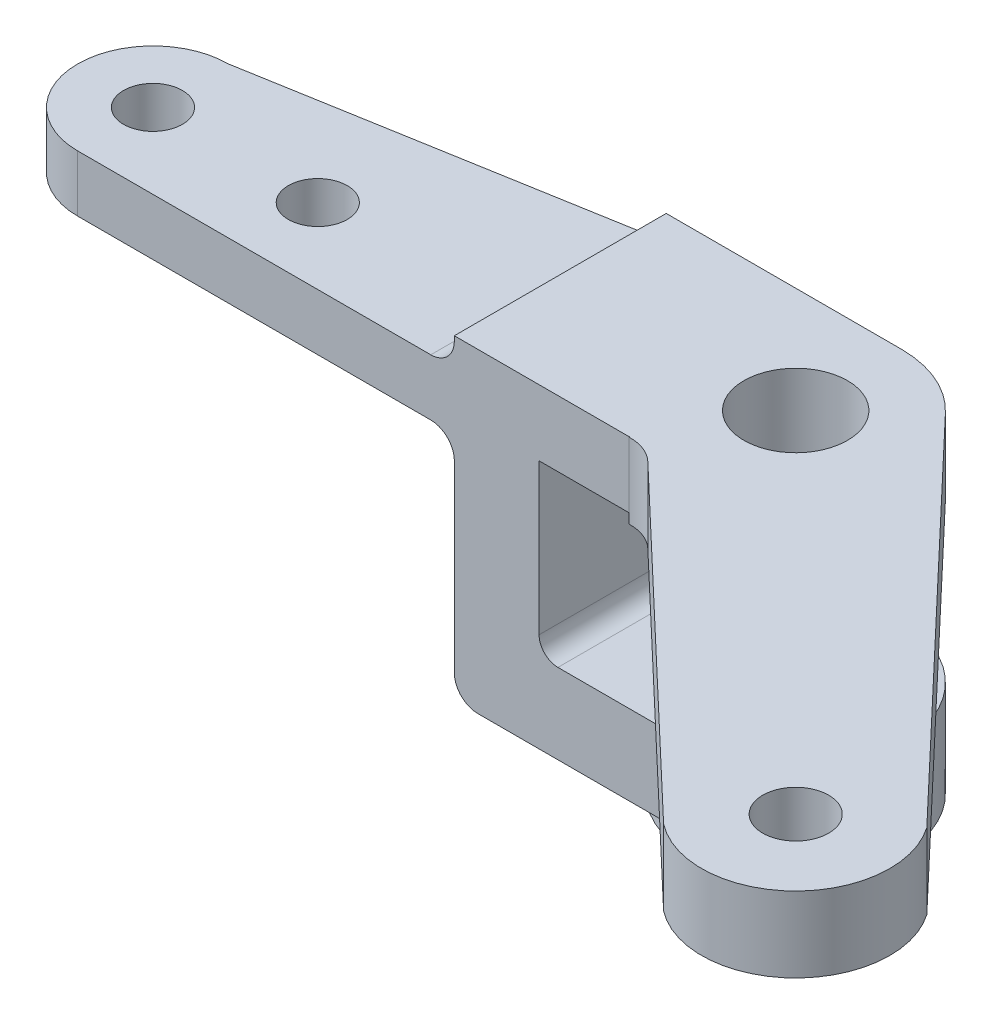
ISO-10303-21;
HEADER;
FILE_DESCRIPTION(('STEP AP214'),'2;1');
FILE_NAME('part.step','',(''),(''),'','','');
FILE_SCHEMA(('AUTOMOTIVE_DESIGN { 1 0 10303 214 1 1 1 1 }'));
ENDSEC;
DATA;
#1=APPLICATION_CONTEXT('core data for automotive mechanical design processes');
#2=APPLICATION_PROTOCOL_DEFINITION('international standard','automotive_design',2000,#1);
#3=PRODUCT_CONTEXT('',#1,'mechanical');
#4=PRODUCT('Part','Part','',(#3));
#5=PRODUCT_RELATED_PRODUCT_CATEGORY('part','',(#4));
#6=PRODUCT_DEFINITION_FORMATION('','',#4);
#7=PRODUCT_DEFINITION_CONTEXT('part definition',#1,'design');
#8=PRODUCT_DEFINITION('design','',#6,#7);
#9=PRODUCT_DEFINITION_SHAPE('','',#8);
#10=(LENGTH_UNIT() NAMED_UNIT(*) SI_UNIT(.MILLI.,.METRE.));
#11=(NAMED_UNIT(*) PLANE_ANGLE_UNIT() SI_UNIT($,.RADIAN.));
#12=(NAMED_UNIT(*) SI_UNIT($,.STERADIAN.) SOLID_ANGLE_UNIT());
#13=UNCERTAINTY_MEASURE_WITH_UNIT(LENGTH_MEASURE(1.E-05),#10,'distance_accuracy_value','');
#14=(GEOMETRIC_REPRESENTATION_CONTEXT(3) GLOBAL_UNCERTAINTY_ASSIGNED_CONTEXT((#13)) GLOBAL_UNIT_ASSIGNED_CONTEXT((#10,
#11,#12)) REPRESENTATION_CONTEXT('',''));
#15=CARTESIAN_POINT('',(0.,0.,0.));
#16=DIRECTION('',(0.,0.,1.));
#17=DIRECTION('',(1.,0.,0.));
#18=AXIS2_PLACEMENT_3D('',#15,#16,#17);
#19=CARTESIAN_POINT('',(130.,-16.,22.5));
#20=DIRECTION('',(0.,1.,0.));
#21=DIRECTION('',(0.,0.,1.));
#22=AXIS2_PLACEMENT_3D('',#19,#20,#21);
#23=PLANE('',#22);
#24=CARTESIAN_POINT('',(204.246212024587,-16.,96.7462120245875));
#25=DIRECTION('',(0.,-1.,0.));
#26=DIRECTION('',(0.,0.,-1.));
#27=AXIS2_PLACEMENT_3D('',#24,#25,#26);
#28=CIRCLE('',#27,6.99999999999999);
#29=CARTESIAN_POINT('',(204.246212024587,-16.,89.7462120245875));
#30=VERTEX_POINT('',#29);
#31=EDGE_CURVE('E445',#30,#30,#28,.T.);
#32=ORIENTED_EDGE('',*,*,#31,.F.);
#33=EDGE_LOOP('',(#32));
#34=FACE_BOUND('',#33,.T.);
#35=CARTESIAN_POINT('',(130.,-16.,22.5));
#36=DIRECTION('',(0.,-1.,0.));
#37=DIRECTION('',(0.,0.,-1.));
#38=AXIS2_PLACEMENT_3D('',#35,#36,#37);
#39=CIRCLE('',#38,22.5);
#40=CARTESIAN_POINT('',(146.71198303914,-16.,7.43482084741492));
#41=VERTEX_POINT('',#40);
#42=CARTESIAN_POINT('',(119.312759657145,-16.,42.2998205510569));
#43=VERTEX_POINT('',#42);
#44=EDGE_CURVE('E200',#41,#43,#39,.T.);
#45=ORIENTED_EDGE('',*,*,#44,.F.);
#46=DIRECTION('',(0.68856588169474,0.,0.725173790595017));
#47=VECTOR('',#46,1.);
#48=CARTESIAN_POINT('',(145.909902576698,-16.,6.5900974233029));
#49=LINE('',#48,#47);
#50=CARTESIAN_POINT('',(220.648460974255,-16.,85.3021642532294));
#51=VERTEX_POINT('',#50);
#52=EDGE_CURVE('E202',#41,#51,#49,.T.);
#53=ORIENTED_EDGE('',*,*,#52,.T.);
#54=CARTESIAN_POINT('',(204.246212024587,-16.,96.746212024588));
#55=DIRECTION('',(0.,-1.,0.));
#56=DIRECTION('',(0.,0.,-1.));
#57=AXIS2_PLACEMENT_3D('',#54,#55,#56);
#58=CIRCLE('',#57,20.);
#59=CARTESIAN_POINT('',(192.010008711411,-16.,112.566304580531));
#60=VERTEX_POINT('',#59);
#61=EDGE_CURVE('E228',#51,#60,#58,.T.);
#62=ORIENTED_EDGE('',*,*,#61,.T.);
#63=DIRECTION('',(-0.724655837018528,0.,-0.689110961946606));
#64=VECTOR('',#63,1.);
#65=CARTESIAN_POINT('',(192.010008711411,-16.,112.566304580531));
#66=LINE('',#65,#64);
#67=CARTESIAN_POINT('',(123.660042494375,-16.,47.5689519577642));
#68=VERTEX_POINT('',#67);
#69=EDGE_CURVE('E226',#60,#68,#66,.T.);
#70=ORIENTED_EDGE('',*,*,#69,.T.);
#71=CARTESIAN_POINT('',(117.458043836856,-16.,54.0908544909309));
#72=DIRECTION('',(0.,1.,0.));
#73=DIRECTION('',(0.,0.,1.));
#74=AXIS2_PLACEMENT_3D('',#71,#72,#73);
#75=CIRCLE('',#74,9.);
#76=CARTESIAN_POINT('',(117.231837637058,-16.,45.0936976758491));
#77=VERTEX_POINT('',#76);
#78=EDGE_CURVE('E229',#68,#77,#75,.T.);
#79=ORIENTED_EDGE('',*,*,#78,.T.);
#80=DIRECTION('',(0.597335430440409,0.,-0.80199151089059));
#81=VECTOR('',#80,1.);
#82=CARTESIAN_POINT('',(117.231837637058,-16.,45.0936976758491));
#83=LINE('',#82,#81);
#84=EDGE_CURVE('E207',#77,#43,#83,.T.);
#85=ORIENTED_EDGE('',*,*,#84,.T.);
#86=EDGE_LOOP('',(#45,#53,#62,#70,#79,#85));
#87=FACE_BOUND('',#86,.T.);
#88=ADVANCED_FACE('F50',(#34,#87),#23,.F.);
#89=CARTESIAN_POINT('',(80.,-50.,45.));
#90=DIRECTION('',(1.,0.,0.));
#91=DIRECTION('',(0.,0.,-1.));
#92=AXIS2_PLACEMENT_3D('',#89,#90,#91);
#93=PLANE('',#92);
#94=DIRECTION('',(0.,-1.,0.));
#95=VECTOR('',#94,1.);
#96=CARTESIAN_POINT('',(80.,-50.,0.));
#97=LINE('',#96,#95);
#98=CARTESIAN_POINT('',(80.,0.,0.));
#99=VERTEX_POINT('',#98);
#100=CARTESIAN_POINT('',(80.,-0.999999999999966,0.));
#101=VERTEX_POINT('',#100);
#102=EDGE_CURVE('E344',#99,#101,#97,.T.);
#103=ORIENTED_EDGE('',*,*,#102,.T.);
#104=DIRECTION('',(0.,0.,1.));
#105=VECTOR('',#104,1.);
#106=CARTESIAN_POINT('',(80.,-0.999999999999964,0.));
#107=LINE('',#106,#105);
#108=CARTESIAN_POINT('',(80.,-0.999999999999966,45.));
#109=VERTEX_POINT('',#108);
#110=EDGE_CURVE('E296',#101,#109,#107,.T.);
#111=ORIENTED_EDGE('',*,*,#110,.T.);
#112=DIRECTION('',(0.,-1.,0.));
#113=VECTOR('',#112,1.);
#114=CARTESIAN_POINT('',(80.,0.,45.));
#115=LINE('',#114,#113);
#116=CARTESIAN_POINT('',(80.,0.,45.));
#117=VERTEX_POINT('',#116);
#118=EDGE_CURVE('E321',#117,#109,#115,.T.);
#119=ORIENTED_EDGE('',*,*,#118,.F.);
#120=DIRECTION('',(0.,0.,-1.));
#121=VECTOR('',#120,1.);
#122=CARTESIAN_POINT('',(80.,0.,45.));
#123=LINE('',#122,#121);
#124=EDGE_CURVE('E11',#117,#99,#123,.T.);
#125=ORIENTED_EDGE('',*,*,#124,.T.);
#126=EDGE_LOOP('',(#103,#111,#119,#125));
#127=FACE_BOUND('',#126,.T.);
#128=ADVANCED_FACE('F414',(#127),#93,.F.);
#129=CARTESIAN_POINT('',(85.,-67.,45.));
#130=DIRECTION('',(0.,1.,0.));
#131=DIRECTION('',(0.,0.,1.));
#132=AXIS2_PLACEMENT_3D('',#129,#130,#131);
#133=PLANE('',#132);
#134=CARTESIAN_POINT('',(130.,-67.,22.5));
#135=DIRECTION('',(0.,-1.,0.));
#136=DIRECTION('',(0.,0.,-1.));
#137=AXIS2_PLACEMENT_3D('',#134,#135,#136);
#138=CIRCLE('',#137,22.5);
#139=CARTESIAN_POINT('',(130.,-67.,45.));
#140=VERTEX_POINT('',#139);
#141=CARTESIAN_POINT('',(130.,-67.,0.));
#142=VERTEX_POINT('',#141);
#143=EDGE_CURVE('E310',#140,#142,#138,.T.);
#144=ORIENTED_EDGE('',*,*,#143,.F.);
#145=DIRECTION('',(1.,0.,0.));
#146=VECTOR('',#145,1.);
#147=CARTESIAN_POINT('',(85.,-67.,45.));
#148=LINE('',#147,#146);
#149=CARTESIAN_POINT('',(85.,-67.,45.));
#150=VERTEX_POINT('',#149);
#151=EDGE_CURVE('E327',#150,#140,#148,.T.);
#152=ORIENTED_EDGE('',*,*,#151,.F.);
#153=DIRECTION('',(0.,0.,-1.));
#154=VECTOR('',#153,1.);
#155=CARTESIAN_POINT('',(85.,-67.,45.));
#156=LINE('',#155,#154);
#157=CARTESIAN_POINT('',(85.,-67.,0.));
#158=VERTEX_POINT('',#157);
#159=EDGE_CURVE('E367',#150,#158,#156,.T.);
#160=ORIENTED_EDGE('',*,*,#159,.T.);
#161=DIRECTION('',(1.,0.,0.));
#162=VECTOR('',#161,1.);
#163=CARTESIAN_POINT('',(85.,-67.,0.));
#164=LINE('',#163,#162);
#165=EDGE_CURVE('E346',#158,#142,#164,.T.);
#166=ORIENTED_EDGE('',*,*,#165,.T.);
#167=EDGE_LOOP('',(#144,#152,#160,#166));
#168=FACE_BOUND('',#167,.T.);
#169=ADVANCED_FACE('F388',(#168),#133,.F.);
#170=CARTESIAN_POINT('',(80.,0.,45.));
#171=DIRECTION('',(0.,-1.,0.));
#172=DIRECTION('',(0.,0.,-1.));
#173=AXIS2_PLACEMENT_3D('',#170,#171,#172);
#174=PLANE('',#173);
#175=CARTESIAN_POINT('',(130.,0.,22.5));
#176=DIRECTION('',(0.,-1.,0.));
#177=DIRECTION('',(0.,0.,-1.));
#178=AXIS2_PLACEMENT_3D('',#175,#176,#177);
#179=CIRCLE('',#178,11.);
#180=CARTESIAN_POINT('',(130.,0.,11.5));
#181=VERTEX_POINT('',#180);
#182=EDGE_CURVE('E444',#181,#181,#179,.T.);
#183=ORIENTED_EDGE('',*,*,#182,.T.);
#184=EDGE_LOOP('',(#183));
#185=FACE_BOUND('',#184,.T.);
#186=CARTESIAN_POINT('',(204.246212024587,0.,96.7462120245875));
#187=DIRECTION('',(0.,-1.,0.));
#188=DIRECTION('',(0.,0.,-1.));
#189=AXIS2_PLACEMENT_3D('',#186,#187,#188);
#190=CIRCLE('',#189,6.99999999999999);
#191=CARTESIAN_POINT('',(204.246212024587,0.,89.7462120245875));
#192=VERTEX_POINT('',#191);
#193=EDGE_CURVE('E208',#192,#192,#190,.T.);
#194=ORIENTED_EDGE('',*,*,#193,.T.);
#195=EDGE_LOOP('',(#194));
#196=FACE_BOUND('',#195,.T.);
#197=DIRECTION('',(-1.,0.,0.));
#198=VECTOR('',#197,1.);
#199=CARTESIAN_POINT('',(80.,0.,45.));
#200=LINE('',#199,#198);
#201=CARTESIAN_POINT('',(117.301625085896,0.,45.));
#202=VERTEX_POINT('',#201);
#203=EDGE_CURVE('E320',#202,#117,#200,.T.);
#204=ORIENTED_EDGE('',*,*,#203,.F.);
#205=DIRECTION('',(0.597335430440409,0.,-0.80199151089059));
#206=VECTOR('',#205,1.);
#207=CARTESIAN_POINT('',(117.231837637058,0.,45.0936976758491));
#208=LINE('',#207,#206);
#209=CARTESIAN_POINT('',(117.231837637058,0.,45.0936976758491));
#210=VERTEX_POINT('',#209);
#211=EDGE_CURVE('E425',#210,#202,#208,.T.);
#212=ORIENTED_EDGE('',*,*,#211,.F.);
#213=CARTESIAN_POINT('',(117.458043836856,0.,54.0908544909309));
#214=DIRECTION('',(0.,1.,0.));
#215=DIRECTION('',(0.,0.,1.));
#216=AXIS2_PLACEMENT_3D('',#213,#214,#215);
#217=CIRCLE('',#216,9.);
#218=CARTESIAN_POINT('',(123.660042494375,0.,47.5689519577642));
#219=VERTEX_POINT('',#218);
#220=EDGE_CURVE('E236',#219,#210,#217,.T.);
#221=ORIENTED_EDGE('',*,*,#220,.F.);
#222=DIRECTION('',(-0.724655837018528,0.,-0.689110961946606));
#223=VECTOR('',#222,1.);
#224=CARTESIAN_POINT('',(192.010008711411,0.,112.566304580531));
#225=LINE('',#224,#223);
#226=CARTESIAN_POINT('',(192.010008711411,0.,112.566304580531));
#227=VERTEX_POINT('',#226);
#228=EDGE_CURVE('E244',#227,#219,#225,.T.);
#229=ORIENTED_EDGE('',*,*,#228,.F.);
#230=CARTESIAN_POINT('',(204.246212024587,0.,96.746212024588));
#231=DIRECTION('',(0.,-1.,0.));
#232=DIRECTION('',(0.,0.,-1.));
#233=AXIS2_PLACEMENT_3D('',#230,#231,#232);
#234=CIRCLE('',#233,20.);
#235=CARTESIAN_POINT('',(220.648460974255,0.,85.3021642532294));
#236=VERTEX_POINT('',#235);
#237=EDGE_CURVE('E429',#236,#227,#234,.T.);
#238=ORIENTED_EDGE('',*,*,#237,.F.);
#239=DIRECTION('',(0.68856588169474,0.,0.725173790595017));
#240=VECTOR('',#239,1.);
#241=CARTESIAN_POINT('',(145.909902576698,0.,6.5900974233029));
#242=LINE('',#241,#240);
#243=CARTESIAN_POINT('',(146.71198303914,0.,7.43482084741494));
#244=VERTEX_POINT('',#243);
#245=EDGE_CURVE('E430',#244,#236,#242,.T.);
#246=ORIENTED_EDGE('',*,*,#245,.F.);
#247=CARTESIAN_POINT('',(130.,0.,22.5));
#248=DIRECTION('',(0.,1.,0.));
#249=DIRECTION('',(0.,0.,1.));
#250=AXIS2_PLACEMENT_3D('',#247,#248,#249);
#251=CIRCLE('',#250,22.5);
#252=CARTESIAN_POINT('',(130.,0.,0.));
#253=VERTEX_POINT('',#252);
#254=EDGE_CURVE('E219',#244,#253,#251,.T.);
#255=ORIENTED_EDGE('',*,*,#254,.T.);
#256=DIRECTION('',(-1.,0.,0.));
#257=VECTOR('',#256,1.);
#258=CARTESIAN_POINT('',(80.,0.,0.));
#259=LINE('',#258,#257);
#260=EDGE_CURVE('E341',#253,#99,#259,.T.);
#261=ORIENTED_EDGE('',*,*,#260,.T.);
#262=ORIENTED_EDGE('',*,*,#124,.F.);
#263=EDGE_LOOP('',(#204,#212,#221,#229,#238,#246,#255,#261,#262));
#264=FACE_BOUND('',#263,.T.);
#265=ADVANCED_FACE('F47',(#185,#196,#264),#174,.F.);
#266=CARTESIAN_POINT('',(80.,-23.,45.));
#267=VERTEX_POINT('',#266);
#268=CARTESIAN_POINT('',(80.,-62.,45.));
#269=VERTEX_POINT('',#268);
#270=EDGE_CURVE('E316',#267,#269,#115,.T.);
#271=ORIENTED_EDGE('',*,*,#270,.F.);
#272=DIRECTION('',(0.,0.,1.));
#273=VECTOR('',#272,1.);
#274=CARTESIAN_POINT('',(80.,-23.,0.));
#275=LINE('',#274,#273);
#276=CARTESIAN_POINT('',(80.,-23.,0.));
#277=VERTEX_POINT('',#276);
#278=EDGE_CURVE('E297',#277,#267,#275,.T.);
#279=ORIENTED_EDGE('',*,*,#278,.F.);
#280=CARTESIAN_POINT('',(80.,-62.,0.));
#281=VERTEX_POINT('',#280);
#282=EDGE_CURVE('E343',#277,#281,#97,.T.);
#283=ORIENTED_EDGE('',*,*,#282,.T.);
#284=DIRECTION('',(0.,0.,-1.));
#285=VECTOR('',#284,1.);
#286=CARTESIAN_POINT('',(80.,-62.,45.));
#287=LINE('',#286,#285);
#288=EDGE_CURVE('E57',#269,#281,#287,.T.);
#289=ORIENTED_EDGE('',*,*,#288,.F.);
#290=EDGE_LOOP('',(#271,#279,#283,#289));
#291=FACE_BOUND('',#290,.T.);
#292=ADVANCED_FACE('F391',(#291),#93,.F.);
#293=CARTESIAN_POINT('',(85.,-62.,45.));
#294=DIRECTION('',(0.,0.,-1.));
#295=DIRECTION('',(-1.,0.,0.));
#296=AXIS2_PLACEMENT_3D('',#293,#294,#295);
#297=CYLINDRICAL_SURFACE('',#296,5.);
#298=CARTESIAN_POINT('',(85.,-62.,0.));
#299=DIRECTION('',(0.,0.,1.));
#300=DIRECTION('',(1.,0.,0.));
#301=AXIS2_PLACEMENT_3D('',#298,#299,#300);
#302=CIRCLE('',#301,5.);
#303=EDGE_CURVE('E349',#281,#158,#302,.T.);
#304=ORIENTED_EDGE('',*,*,#303,.T.);
#305=ORIENTED_EDGE('',*,*,#159,.F.);
#306=CARTESIAN_POINT('',(85.,-62.,45.));
#307=DIRECTION('',(0.,0.,1.));
#308=DIRECTION('',(1.,0.,0.));
#309=AXIS2_PLACEMENT_3D('',#306,#307,#308);
#310=CIRCLE('',#309,5.);
#311=EDGE_CURVE('E323',#269,#150,#310,.T.);
#312=ORIENTED_EDGE('',*,*,#311,.F.);
#313=ORIENTED_EDGE('',*,*,#288,.T.);
#314=EDGE_LOOP('',(#304,#305,#312,#313));
#315=FACE_BOUND('',#314,.T.);
#316=ADVANCED_FACE('F380',(#315),#297,.T.);
#317=CARTESIAN_POINT('',(102.,-50.,45.));
#318=DIRECTION('',(0.,-1.,0.));
#319=DIRECTION('',(0.,0.,-1.));
#320=AXIS2_PLACEMENT_3D('',#317,#318,#319);
#321=PLANE('',#320);
#322=CARTESIAN_POINT('',(130.,-50.,22.5));
#323=DIRECTION('',(0.,-1.,0.));
#324=DIRECTION('',(0.,0.,-1.));
#325=AXIS2_PLACEMENT_3D('',#322,#323,#324);
#326=CIRCLE('',#325,11.);
#327=CARTESIAN_POINT('',(130.,-50.,11.5));
#328=VERTEX_POINT('',#327);
#329=EDGE_CURVE('E448',#328,#328,#326,.T.);
#330=ORIENTED_EDGE('',*,*,#329,.T.);
#331=EDGE_LOOP('',(#330));
#332=FACE_BOUND('',#331,.T.);
#333=DIRECTION('',(-1.,0.,0.));
#334=VECTOR('',#333,1.);
#335=CARTESIAN_POINT('',(102.,-50.,45.));
#336=LINE('',#335,#334);
#337=CARTESIAN_POINT('',(130.,-50.,45.));
#338=VERTEX_POINT('',#337);
#339=CARTESIAN_POINT('',(102.,-50.,45.));
#340=VERTEX_POINT('',#339);
#341=EDGE_CURVE('E331',#338,#340,#336,.T.);
#342=ORIENTED_EDGE('',*,*,#341,.F.);
#343=CARTESIAN_POINT('',(130.,-50.,22.5));
#344=DIRECTION('',(0.,-1.,0.));
#345=DIRECTION('',(0.,0.,-1.));
#346=AXIS2_PLACEMENT_3D('',#343,#344,#345);
#347=CIRCLE('',#346,22.5);
#348=CARTESIAN_POINT('',(130.,-50.,0.));
#349=VERTEX_POINT('',#348);
#350=EDGE_CURVE('E311',#349,#338,#347,.T.);
#351=ORIENTED_EDGE('',*,*,#350,.F.);
#352=DIRECTION('',(-1.,0.,0.));
#353=VECTOR('',#352,1.);
#354=CARTESIAN_POINT('',(102.,-50.,0.));
#355=LINE('',#354,#353);
#356=CARTESIAN_POINT('',(102.,-50.,0.));
#357=VERTEX_POINT('',#356);
#358=EDGE_CURVE('E353',#349,#357,#355,.T.);
#359=ORIENTED_EDGE('',*,*,#358,.T.);
#360=DIRECTION('',(0.,0.,-1.));
#361=VECTOR('',#360,1.);
#362=CARTESIAN_POINT('',(102.,-50.,45.));
#363=LINE('',#362,#361);
#364=EDGE_CURVE('E366',#340,#357,#363,.T.);
#365=ORIENTED_EDGE('',*,*,#364,.F.);
#366=EDGE_LOOP('',(#342,#351,#359,#365));
#367=FACE_BOUND('',#366,.T.);
#368=ADVANCED_FACE('F514',(#332,#367),#321,.F.);
#369=CARTESIAN_POINT('',(102.,-46.,45.));
#370=DIRECTION('',(0.,0.,-1.));
#371=DIRECTION('',(-1.,0.,0.));
#372=AXIS2_PLACEMENT_3D('',#369,#370,#371);
#373=CYLINDRICAL_SURFACE('',#372,4.);
#374=CARTESIAN_POINT('',(102.,-46.,0.));
#375=DIRECTION('',(0.,0.,-1.));
#376=DIRECTION('',(-1.,0.,0.));
#377=AXIS2_PLACEMENT_3D('',#374,#375,#376);
#378=CIRCLE('',#377,4.);
#379=CARTESIAN_POINT('',(98.,-46.,0.));
#380=VERTEX_POINT('',#379);
#381=EDGE_CURVE('E358',#357,#380,#378,.T.);
#382=ORIENTED_EDGE('',*,*,#381,.T.);
#383=DIRECTION('',(0.,0.,-1.));
#384=VECTOR('',#383,1.);
#385=CARTESIAN_POINT('',(98.,-46.,45.));
#386=LINE('',#385,#384);
#387=CARTESIAN_POINT('',(98.,-46.,45.));
#388=VERTEX_POINT('',#387);
#389=EDGE_CURVE('E361',#388,#380,#386,.T.);
#390=ORIENTED_EDGE('',*,*,#389,.F.);
#391=CARTESIAN_POINT('',(102.,-46.,45.));
#392=DIRECTION('',(0.,0.,-1.));
#393=DIRECTION('',(-1.,0.,0.));
#394=AXIS2_PLACEMENT_3D('',#391,#392,#393);
#395=CIRCLE('',#394,4.);
#396=EDGE_CURVE('E334',#340,#388,#395,.T.);
#397=ORIENTED_EDGE('',*,*,#396,.F.);
#398=ORIENTED_EDGE('',*,*,#364,.T.);
#399=EDGE_LOOP('',(#382,#390,#397,#398));
#400=FACE_BOUND('',#399,.T.);
#401=ADVANCED_FACE('F508',(#400),#373,.F.);
#402=CARTESIAN_POINT('',(98.,-14.,45.));
#403=DIRECTION('',(-1.,0.,0.));
#404=DIRECTION('',(0.,0.,1.));
#405=AXIS2_PLACEMENT_3D('',#402,#403,#404);
#406=PLANE('',#405);
#407=DIRECTION('',(0.,1.,0.));
#408=VECTOR('',#407,1.);
#409=CARTESIAN_POINT('',(98.,-14.,0.));
#410=LINE('',#409,#408);
#411=CARTESIAN_POINT('',(98.,-14.,0.));
#412=VERTEX_POINT('',#411);
#413=EDGE_CURVE('E356',#380,#412,#410,.T.);
#414=ORIENTED_EDGE('',*,*,#413,.T.);
#415=DIRECTION('',(0.,0.,-1.));
#416=VECTOR('',#415,1.);
#417=CARTESIAN_POINT('',(98.,-14.,45.));
#418=LINE('',#417,#416);
#419=CARTESIAN_POINT('',(98.,-14.,45.));
#420=VERTEX_POINT('',#419);
#421=EDGE_CURVE('E339',#420,#412,#418,.T.);
#422=ORIENTED_EDGE('',*,*,#421,.F.);
#423=DIRECTION('',(0.,1.,0.));
#424=VECTOR('',#423,1.);
#425=CARTESIAN_POINT('',(98.,-14.,45.));
#426=LINE('',#425,#424);
#427=EDGE_CURVE('E335',#388,#420,#426,.T.);
#428=ORIENTED_EDGE('',*,*,#427,.F.);
#429=ORIENTED_EDGE('',*,*,#389,.T.);
#430=EDGE_LOOP('',(#414,#422,#428,#429));
#431=FACE_BOUND('',#430,.T.);
#432=ADVANCED_FACE('F506',(#431),#406,.F.);
#433=CARTESIAN_POINT('',(130.,-14.,45.));
#434=DIRECTION('',(0.,1.,0.));
#435=DIRECTION('',(0.,0.,1.));
#436=AXIS2_PLACEMENT_3D('',#433,#434,#435);
#437=PLANE('',#436);
#438=CARTESIAN_POINT('',(130.,-14.,22.5));
#439=DIRECTION('',(0.,1.,0.));
#440=DIRECTION('',(0.,0.,1.));
#441=AXIS2_PLACEMENT_3D('',#438,#439,#440);
#442=CIRCLE('',#441,22.5);
#443=CARTESIAN_POINT('',(130.,-14.,0.));
#444=VERTEX_POINT('',#443);
#445=CARTESIAN_POINT('',(119.312759657145,-14.,42.2998205510569));
#446=VERTEX_POINT('',#445);
#447=EDGE_CURVE('E304',#444,#446,#442,.T.);
#448=ORIENTED_EDGE('',*,*,#447,.T.);
#449=DIRECTION('',(-0.597335430440409,0.,0.80199151089059));
#450=VECTOR('',#449,1.);
#451=CARTESIAN_POINT('',(121.832527368655,-14.,38.9167426168427));
#452=LINE('',#451,#450);
#453=CARTESIAN_POINT('',(117.301625085896,-14.,45.));
#454=VERTEX_POINT('',#453);
#455=EDGE_CURVE('E62',#446,#454,#452,.T.);
#456=ORIENTED_EDGE('',*,*,#455,.T.);
#457=DIRECTION('',(1.,0.,0.));
#458=VECTOR('',#457,1.);
#459=CARTESIAN_POINT('',(130.,-14.,45.));
#460=LINE('',#459,#458);
#461=EDGE_CURVE('E340',#420,#454,#460,.T.);
#462=ORIENTED_EDGE('',*,*,#461,.F.);
#463=ORIENTED_EDGE('',*,*,#421,.T.);
#464=DIRECTION('',(1.,0.,0.));
#465=VECTOR('',#464,1.);
#466=CARTESIAN_POINT('',(130.,-14.,0.));
#467=LINE('',#466,#465);
#468=EDGE_CURVE('E318',#412,#444,#467,.T.);
#469=ORIENTED_EDGE('',*,*,#468,.T.);
#470=EDGE_LOOP('',(#448,#456,#462,#463,#469));
#471=FACE_BOUND('',#470,.T.);
#472=ADVANCED_FACE('F423',(#471),#437,.F.);
#473=CARTESIAN_POINT('',(102.,-46.,45.));
#474=DIRECTION('',(0.,0.,-1.));
#475=DIRECTION('',(-1.,0.,0.));
#476=AXIS2_PLACEMENT_3D('',#473,#474,#475);
#477=PLANE('',#476);
#478=ORIENTED_EDGE('',*,*,#461,.T.);
#479=DIRECTION('',(0.,1.,0.));
#480=VECTOR('',#479,1.);
#481=CARTESIAN_POINT('',(117.301625085896,-46.,45.));
#482=LINE('',#481,#480);
#483=EDGE_CURVE('E68',#454,#202,#482,.T.);
#484=ORIENTED_EDGE('',*,*,#483,.T.);
#485=ORIENTED_EDGE('',*,*,#203,.T.);
#486=ORIENTED_EDGE('',*,*,#118,.T.);
#487=CARTESIAN_POINT('',(75.,-1.,45.));
#488=DIRECTION('',(0.,0.,1.));
#489=DIRECTION('',(1.,0.,0.));
#490=AXIS2_PLACEMENT_3D('',#487,#488,#489);
#491=CIRCLE('',#490,5.);
#492=CARTESIAN_POINT('',(75.,-6.,45.));
#493=VERTEX_POINT('',#492);
#494=EDGE_CURVE('E290',#493,#109,#491,.T.);
#495=ORIENTED_EDGE('',*,*,#494,.F.);
#496=DIRECTION('',(-1.,0.,0.));
#497=VECTOR('',#496,1.);
#498=CARTESIAN_POINT('',(0.,-6.,45.));
#499=LINE('',#498,#497);
#500=CARTESIAN_POINT('',(0.,-6.,45.));
#501=VERTEX_POINT('',#500);
#502=EDGE_CURVE('E291',#493,#501,#499,.T.);
#503=ORIENTED_EDGE('',*,*,#502,.T.);
#504=DIRECTION('',(0.,-1.,0.));
#505=VECTOR('',#504,1.);
#506=CARTESIAN_POINT('',(0.,0.,45.));
#507=LINE('',#506,#505);
#508=CARTESIAN_POINT('',(0.,-18.,45.));
#509=VERTEX_POINT('',#508);
#510=EDGE_CURVE('E282',#501,#509,#507,.T.);
#511=ORIENTED_EDGE('',*,*,#510,.T.);
#512=DIRECTION('',(1.,0.,0.));
#513=VECTOR('',#512,1.);
#514=CARTESIAN_POINT('',(0.,-18.,45.));
#515=LINE('',#514,#513);
#516=CARTESIAN_POINT('',(75.,-18.,45.));
#517=VERTEX_POINT('',#516);
#518=EDGE_CURVE('E276',#509,#517,#515,.T.);
#519=ORIENTED_EDGE('',*,*,#518,.T.);
#520=CARTESIAN_POINT('',(75.,-23.,45.));
#521=DIRECTION('',(0.,0.,1.));
#522=DIRECTION('',(1.,0.,0.));
#523=AXIS2_PLACEMENT_3D('',#520,#521,#522);
#524=CIRCLE('',#523,5.);
#525=EDGE_CURVE('E287',#517,#267,#524,.F.);
#526=ORIENTED_EDGE('',*,*,#525,.T.);
#527=ORIENTED_EDGE('',*,*,#270,.T.);
#528=ORIENTED_EDGE('',*,*,#311,.T.);
#529=ORIENTED_EDGE('',*,*,#151,.T.);
#530=DIRECTION('',(0.,1.,0.));
#531=VECTOR('',#530,1.);
#532=CARTESIAN_POINT('',(130.,-67.,45.));
#533=LINE('',#532,#531);
#534=EDGE_CURVE('E326',#140,#338,#533,.T.);
#535=ORIENTED_EDGE('',*,*,#534,.T.);
#536=ORIENTED_EDGE('',*,*,#341,.T.);
#537=ORIENTED_EDGE('',*,*,#396,.T.);
#538=ORIENTED_EDGE('',*,*,#427,.T.);
#539=EDGE_LOOP('',(#478,#484,#485,#486,#495,#503,#511,#519,#526,#527,#528,#529,#535,#536,#537,#538));
#540=FACE_BOUND('',#539,.T.);
#541=ADVANCED_FACE('F392',(#540),#477,.F.);
#542=CARTESIAN_POINT('',(102.,-46.,0.));
#543=DIRECTION('',(0.,0.,-1.));
#544=DIRECTION('',(-1.,0.,0.));
#545=AXIS2_PLACEMENT_3D('',#542,#543,#544);
#546=PLANE('',#545);
#547=DIRECTION('',(0.,-1.,0.));
#548=VECTOR('',#547,1.);
#549=CARTESIAN_POINT('',(75.,-6.,0.));
#550=LINE('',#549,#548);
#551=CARTESIAN_POINT('',(75.,-6.,0.));
#552=VERTEX_POINT('',#551);
#553=CARTESIAN_POINT('',(75.,-18.,0.));
#554=VERTEX_POINT('',#553);
#555=EDGE_CURVE('E261',#552,#554,#550,.T.);
#556=ORIENTED_EDGE('',*,*,#555,.F.);
#557=CARTESIAN_POINT('',(75.,-1.,0.));
#558=DIRECTION('',(0.,0.,1.));
#559=DIRECTION('',(1.,0.,0.));
#560=AXIS2_PLACEMENT_3D('',#557,#558,#559);
#561=CIRCLE('',#560,5.);
#562=EDGE_CURVE('E279',#552,#101,#561,.T.);
#563=ORIENTED_EDGE('',*,*,#562,.T.);
#564=ORIENTED_EDGE('',*,*,#102,.F.);
#565=ORIENTED_EDGE('',*,*,#260,.F.);
#566=DIRECTION('',(0.,1.,0.));
#567=VECTOR('',#566,1.);
#568=CARTESIAN_POINT('',(130.,0.,0.));
#569=LINE('',#568,#567);
#570=EDGE_CURVE('E317',#444,#253,#569,.T.);
#571=ORIENTED_EDGE('',*,*,#570,.F.);
#572=ORIENTED_EDGE('',*,*,#468,.F.);
#573=ORIENTED_EDGE('',*,*,#413,.F.);
#574=ORIENTED_EDGE('',*,*,#381,.F.);
#575=ORIENTED_EDGE('',*,*,#358,.F.);
#576=DIRECTION('',(0.,1.,0.));
#577=VECTOR('',#576,1.);
#578=CARTESIAN_POINT('',(130.,-67.,0.));
#579=LINE('',#578,#577);
#580=EDGE_CURVE('E351',#142,#349,#579,.T.);
#581=ORIENTED_EDGE('',*,*,#580,.F.);
#582=ORIENTED_EDGE('',*,*,#165,.F.);
#583=ORIENTED_EDGE('',*,*,#303,.F.);
#584=ORIENTED_EDGE('',*,*,#282,.F.);
#585=CARTESIAN_POINT('',(75.,-23.,0.));
#586=DIRECTION('',(0.,0.,1.));
#587=DIRECTION('',(1.,0.,0.));
#588=AXIS2_PLACEMENT_3D('',#585,#586,#587);
#589=CIRCLE('',#588,5.);
#590=EDGE_CURVE('E280',#554,#277,#589,.F.);
#591=ORIENTED_EDGE('',*,*,#590,.F.);
#592=EDGE_LOOP('',(#556,#563,#564,#565,#571,#572,#573,#574,#575,#581,#582,#583,#584,#591));
#593=FACE_BOUND('',#592,.T.);
#594=ADVANCED_FACE('F384',(#593),#546,.T.);
#595=CARTESIAN_POINT('',(130.,-50.,22.5));
#596=DIRECTION('',(0.,-1.,0.));
#597=DIRECTION('',(0.,0.,-1.));
#598=AXIS2_PLACEMENT_3D('',#595,#596,#597);
#599=CYLINDRICAL_SURFACE('',#598,22.5);
#600=ORIENTED_EDGE('',*,*,#350,.T.);
#601=ORIENTED_EDGE('',*,*,#534,.F.);
#602=ORIENTED_EDGE('',*,*,#143,.T.);
#603=ORIENTED_EDGE('',*,*,#580,.T.);
#604=EDGE_LOOP('',(#600,#601,#602,#603));
#605=FACE_BOUND('',#604,.T.);
#606=CARTESIAN_POINT('',(130.,-70.5,22.5));
#607=DIRECTION('',(0.,-1.,0.));
#608=DIRECTION('',(0.,0.,-1.));
#609=AXIS2_PLACEMENT_3D('',#606,#607,#608);
#610=CIRCLE('',#609,22.5);
#611=CARTESIAN_POINT('',(130.,-70.5,0.));
#612=VERTEX_POINT('',#611);
#613=EDGE_CURVE('E308',#612,#612,#610,.T.);
#614=ORIENTED_EDGE('',*,*,#613,.F.);
#615=EDGE_LOOP('',(#614));
#616=FACE_BOUND('',#615,.T.);
#617=ADVANCED_FACE('F492',(#605,#616),#599,.T.);
#618=CARTESIAN_POINT('',(130.,-70.5,22.5));
#619=DIRECTION('',(0.,-1.,0.));
#620=DIRECTION('',(0.,0.,-1.));
#621=AXIS2_PLACEMENT_3D('',#618,#619,#620);
#622=PLANE('',#621);
#623=CARTESIAN_POINT('',(130.,-70.5,22.5));
#624=DIRECTION('',(0.,-1.,0.));
#625=DIRECTION('',(0.,0.,-1.));
#626=AXIS2_PLACEMENT_3D('',#623,#624,#625);
#627=CIRCLE('',#626,11.);
#628=CARTESIAN_POINT('',(130.,-70.5,11.5));
#629=VERTEX_POINT('',#628);
#630=EDGE_CURVE('E452',#629,#629,#627,.T.);
#631=ORIENTED_EDGE('',*,*,#630,.F.);
#632=EDGE_LOOP('',(#631));
#633=FACE_BOUND('',#632,.T.);
#634=ORIENTED_EDGE('',*,*,#613,.T.);
#635=EDGE_LOOP('',(#634));
#636=FACE_BOUND('',#635,.T.);
#637=ADVANCED_FACE('F495',(#633,#636),#622,.T.);
#638=CARTESIAN_POINT('',(130.,-16.,22.5));
#639=DIRECTION('',(0.,1.,0.));
#640=DIRECTION('',(0.,0.,1.));
#641=AXIS2_PLACEMENT_3D('',#638,#639,#640);
#642=CYLINDRICAL_SURFACE('',#641,22.5);
#643=DIRECTION('',(0.,1.,0.));
#644=VECTOR('',#643,1.);
#645=CARTESIAN_POINT('',(119.312759657145,-16.,42.2998205510569));
#646=LINE('',#645,#644);
#647=EDGE_CURVE('E237',#446,#43,#646,.F.);
#648=ORIENTED_EDGE('',*,*,#647,.F.);
#649=ORIENTED_EDGE('',*,*,#447,.F.);
#650=ORIENTED_EDGE('',*,*,#570,.T.);
#651=ORIENTED_EDGE('',*,*,#254,.F.);
#652=DIRECTION('',(0.,1.,0.));
#653=VECTOR('',#652,1.);
#654=CARTESIAN_POINT('',(146.71198303914,-16.,7.43482084741486));
#655=LINE('',#654,#653);
#656=EDGE_CURVE('E212',#41,#244,#655,.T.);
#657=ORIENTED_EDGE('',*,*,#656,.F.);
#658=ORIENTED_EDGE('',*,*,#44,.T.);
#659=EDGE_LOOP('',(#648,#649,#650,#651,#657,#658));
#660=FACE_BOUND('',#659,.T.);
#661=CARTESIAN_POINT('',(130.,-17.,22.5));
#662=DIRECTION('',(0.,-1.,0.));
#663=DIRECTION('',(0.,0.,-1.));
#664=AXIS2_PLACEMENT_3D('',#661,#662,#663);
#665=CIRCLE('',#664,22.5);
#666=CARTESIAN_POINT('',(130.,-17.,0.));
#667=VERTEX_POINT('',#666);
#668=EDGE_CURVE('E209',#667,#667,#665,.T.);
#669=ORIENTED_EDGE('',*,*,#668,.F.);
#670=EDGE_LOOP('',(#669));
#671=FACE_BOUND('',#670,.T.);
#672=ADVANCED_FACE('F213',(#660,#671),#642,.T.);
#673=CARTESIAN_POINT('',(0.,-18.,0.));
#674=DIRECTION('',(0.,-1.,0.));
#675=DIRECTION('',(0.,0.,-1.));
#676=AXIS2_PLACEMENT_3D('',#673,#674,#675);
#677=PLANE('',#676);
#678=CARTESIAN_POINT('',(0.,-18.,29.));
#679=DIRECTION('',(0.,-1.,0.));
#680=DIRECTION('',(0.,0.,-1.));
#681=AXIS2_PLACEMENT_3D('',#678,#679,#680);
#682=CIRCLE('',#681,6.25);
#683=CARTESIAN_POINT('',(0.,-18.,22.75));
#684=VERTEX_POINT('',#683);
#685=EDGE_CURVE('E254',#684,#684,#682,.T.);
#686=ORIENTED_EDGE('',*,*,#685,.F.);
#687=EDGE_LOOP('',(#686));
#688=FACE_BOUND('',#687,.T.);
#689=CARTESIAN_POINT('',(35.,-18.,29.));
#690=DIRECTION('',(0.,-1.,0.));
#691=DIRECTION('',(0.,0.,-1.));
#692=AXIS2_PLACEMENT_3D('',#689,#690,#691);
#693=CIRCLE('',#692,6.25000000000001);
#694=CARTESIAN_POINT('',(35.,-18.,22.75));
#695=VERTEX_POINT('',#694);
#696=EDGE_CURVE('E218',#695,#695,#693,.T.);
#697=ORIENTED_EDGE('',*,*,#696,.F.);
#698=EDGE_LOOP('',(#697));
#699=FACE_BOUND('',#698,.T.);
#700=DIRECTION('',(-0.985308020399641,0.,0.170786723535938));
#701=VECTOR('',#700,1.);
#702=CARTESIAN_POINT('',(75.,-18.,0.));
#703=LINE('',#702,#701);
#704=CARTESIAN_POINT('',(0.,-18.,13.));
#705=VERTEX_POINT('',#704);
#706=EDGE_CURVE('E255',#554,#705,#703,.T.);
#707=ORIENTED_EDGE('',*,*,#706,.F.);
#708=DIRECTION('',(0.,0.,1.));
#709=VECTOR('',#708,1.);
#710=CARTESIAN_POINT('',(75.,-18.,0.));
#711=LINE('',#710,#709);
#712=EDGE_CURVE('E281',#554,#517,#711,.T.);
#713=ORIENTED_EDGE('',*,*,#712,.T.);
#714=ORIENTED_EDGE('',*,*,#518,.F.);
#715=CARTESIAN_POINT('',(0.,-18.,29.));
#716=DIRECTION('',(0.,-1.,0.));
#717=DIRECTION('',(0.,0.,-1.));
#718=AXIS2_PLACEMENT_3D('',#715,#716,#717);
#719=CIRCLE('',#718,16.);
#720=EDGE_CURVE('E267',#509,#705,#719,.T.);
#721=ORIENTED_EDGE('',*,*,#720,.T.);
#722=EDGE_LOOP('',(#707,#713,#714,#721));
#723=FACE_BOUND('',#722,.T.);
#724=ADVANCED_FACE('F486',(#688,#699,#723),#677,.T.);
#725=CARTESIAN_POINT('',(0.,-6.,0.));
#726=DIRECTION('',(0.,1.,0.));
#727=DIRECTION('',(0.,0.,1.));
#728=AXIS2_PLACEMENT_3D('',#725,#726,#727);
#729=PLANE('',#728);
#730=CARTESIAN_POINT('',(0.,-6.,29.));
#731=DIRECTION('',(0.,-1.,0.));
#732=DIRECTION('',(0.,0.,-1.));
#733=AXIS2_PLACEMENT_3D('',#730,#731,#732);
#734=CIRCLE('',#733,6.25);
#735=CARTESIAN_POINT('',(0.,-6.,22.75));
#736=VERTEX_POINT('',#735);
#737=EDGE_CURVE('E248',#736,#736,#734,.T.);
#738=ORIENTED_EDGE('',*,*,#737,.T.);
#739=EDGE_LOOP('',(#738));
#740=FACE_BOUND('',#739,.T.);
#741=CARTESIAN_POINT('',(35.,-6.,29.));
#742=DIRECTION('',(0.,-1.,0.));
#743=DIRECTION('',(0.,0.,-1.));
#744=AXIS2_PLACEMENT_3D('',#741,#742,#743);
#745=CIRCLE('',#744,6.25000000000001);
#746=CARTESIAN_POINT('',(35.,-6.,22.75));
#747=VERTEX_POINT('',#746);
#748=EDGE_CURVE('E256',#747,#747,#745,.T.);
#749=ORIENTED_EDGE('',*,*,#748,.T.);
#750=EDGE_LOOP('',(#749));
#751=FACE_BOUND('',#750,.T.);
#752=DIRECTION('',(-0.985308020399641,0.,0.170786723535938));
#753=VECTOR('',#752,1.);
#754=CARTESIAN_POINT('',(75.,-6.,0.));
#755=LINE('',#754,#753);
#756=CARTESIAN_POINT('',(0.,-6.,13.));
#757=VERTEX_POINT('',#756);
#758=EDGE_CURVE('E262',#552,#757,#755,.T.);
#759=ORIENTED_EDGE('',*,*,#758,.T.);
#760=CARTESIAN_POINT('',(0.,-6.,29.));
#761=DIRECTION('',(0.,-1.,0.));
#762=DIRECTION('',(0.,0.,-1.));
#763=AXIS2_PLACEMENT_3D('',#760,#761,#762);
#764=CIRCLE('',#763,16.);
#765=EDGE_CURVE('E269',#501,#757,#764,.T.);
#766=ORIENTED_EDGE('',*,*,#765,.F.);
#767=ORIENTED_EDGE('',*,*,#502,.F.);
#768=DIRECTION('',(0.,0.,1.));
#769=VECTOR('',#768,1.);
#770=CARTESIAN_POINT('',(75.,-6.,0.));
#771=LINE('',#770,#769);
#772=EDGE_CURVE('E298',#552,#493,#771,.T.);
#773=ORIENTED_EDGE('',*,*,#772,.F.);
#774=EDGE_LOOP('',(#759,#766,#767,#773));
#775=FACE_BOUND('',#774,.T.);
#776=ADVANCED_FACE('F403',(#740,#751,#775),#729,.T.);
#777=CARTESIAN_POINT('',(75.,-1.,0.));
#778=DIRECTION('',(0.,0.,1.));
#779=DIRECTION('',(1.,0.,0.));
#780=AXIS2_PLACEMENT_3D('',#777,#778,#779);
#781=CYLINDRICAL_SURFACE('',#780,5.);
#782=ORIENTED_EDGE('',*,*,#494,.T.);
#783=ORIENTED_EDGE('',*,*,#110,.F.);
#784=ORIENTED_EDGE('',*,*,#562,.F.);
#785=ORIENTED_EDGE('',*,*,#772,.T.);
#786=EDGE_LOOP('',(#782,#783,#784,#785));
#787=FACE_BOUND('',#786,.T.);
#788=ADVANCED_FACE('F408',(#787),#781,.F.);
#789=CARTESIAN_POINT('',(75.,-23.,0.));
#790=DIRECTION('',(0.,0.,1.));
#791=DIRECTION('',(1.,0.,0.));
#792=AXIS2_PLACEMENT_3D('',#789,#790,#791);
#793=CYLINDRICAL_SURFACE('',#792,5.);
#794=ORIENTED_EDGE('',*,*,#525,.F.);
#795=ORIENTED_EDGE('',*,*,#712,.F.);
#796=ORIENTED_EDGE('',*,*,#590,.T.);
#797=ORIENTED_EDGE('',*,*,#278,.T.);
#798=EDGE_LOOP('',(#794,#795,#796,#797));
#799=FACE_BOUND('',#798,.T.);
#800=ADVANCED_FACE('F396',(#799),#793,.F.);
#801=CARTESIAN_POINT('',(0.,-6.,29.));
#802=DIRECTION('',(0.,-1.,0.));
#803=DIRECTION('',(0.,0.,-1.));
#804=AXIS2_PLACEMENT_3D('',#801,#802,#803);
#805=CYLINDRICAL_SURFACE('',#804,16.);
#806=ORIENTED_EDGE('',*,*,#765,.T.);
#807=DIRECTION('',(0.,-1.,0.));
#808=VECTOR('',#807,1.);
#809=CARTESIAN_POINT('',(0.,-6.,13.));
#810=LINE('',#809,#808);
#811=EDGE_CURVE('E272',#757,#705,#810,.T.);
#812=ORIENTED_EDGE('',*,*,#811,.T.);
#813=ORIENTED_EDGE('',*,*,#720,.F.);
#814=ORIENTED_EDGE('',*,*,#510,.F.);
#815=EDGE_LOOP('',(#806,#812,#813,#814));
#816=FACE_BOUND('',#815,.T.);
#817=ADVANCED_FACE('F746',(#816),#805,.T.);
#818=CARTESIAN_POINT('',(75.,-6.,0.));
#819=DIRECTION('',(0.170786723535938,0.,0.985308020399641));
#820=DIRECTION('',(0.985308020399641,0.,-0.170786723535938));
#821=AXIS2_PLACEMENT_3D('',#818,#819,#820);
#822=PLANE('',#821);
#823=ORIENTED_EDGE('',*,*,#706,.T.);
#824=ORIENTED_EDGE('',*,*,#811,.F.);
#825=ORIENTED_EDGE('',*,*,#758,.F.);
#826=ORIENTED_EDGE('',*,*,#555,.T.);
#827=EDGE_LOOP('',(#823,#824,#825,#826));
#828=FACE_BOUND('',#827,.T.);
#829=ADVANCED_FACE('F592',(#828),#822,.F.);
#830=CARTESIAN_POINT('',(35.,-6.,29.));
#831=DIRECTION('',(0.,-1.,0.));
#832=DIRECTION('',(0.,0.,-1.));
#833=AXIS2_PLACEMENT_3D('',#830,#831,#832);
#834=CYLINDRICAL_SURFACE('',#833,6.25000000000001);
#835=ORIENTED_EDGE('',*,*,#748,.F.);
#836=EDGE_LOOP('',(#835));
#837=FACE_BOUND('',#836,.T.);
#838=ORIENTED_EDGE('',*,*,#696,.T.);
#839=EDGE_LOOP('',(#838));
#840=FACE_BOUND('',#839,.T.);
#841=ADVANCED_FACE('F585',(#837,#840),#834,.F.);
#842=CARTESIAN_POINT('',(0.,-6.,29.));
#843=DIRECTION('',(0.,-1.,0.));
#844=DIRECTION('',(0.,0.,-1.));
#845=AXIS2_PLACEMENT_3D('',#842,#843,#844);
#846=CYLINDRICAL_SURFACE('',#845,6.25);
#847=ORIENTED_EDGE('',*,*,#737,.F.);
#848=EDGE_LOOP('',(#847));
#849=FACE_BOUND('',#848,.T.);
#850=ORIENTED_EDGE('',*,*,#685,.T.);
#851=EDGE_LOOP('',(#850));
#852=FACE_BOUND('',#851,.T.);
#853=ADVANCED_FACE('F579',(#849,#852),#846,.F.);
#854=CARTESIAN_POINT('',(117.231837637058,0.,45.0936976758491));
#855=DIRECTION('',(-0.80199151089059,0.,-0.597335430440409));
#856=DIRECTION('',(-0.597335430440409,0.,0.80199151089059));
#857=AXIS2_PLACEMENT_3D('',#854,#855,#856);
#858=PLANE('',#857);
#859=ORIENTED_EDGE('',*,*,#483,.F.);
#860=ORIENTED_EDGE('',*,*,#455,.F.);
#861=ORIENTED_EDGE('',*,*,#647,.T.);
#862=ORIENTED_EDGE('',*,*,#84,.F.);
#863=DIRECTION('',(0.,-1.,0.));
#864=VECTOR('',#863,1.);
#865=CARTESIAN_POINT('',(117.231837637058,0.,45.0936976758491));
#866=LINE('',#865,#864);
#867=EDGE_CURVE('E243',#210,#77,#866,.T.);
#868=ORIENTED_EDGE('',*,*,#867,.F.);
#869=ORIENTED_EDGE('',*,*,#211,.T.);
#870=EDGE_LOOP('',(#859,#860,#861,#862,#868,#869));
#871=FACE_BOUND('',#870,.T.);
#872=ADVANCED_FACE('F421',(#871),#858,.T.);
#873=CARTESIAN_POINT('',(117.458043836856,0.,54.0908544909309));
#874=DIRECTION('',(0.,-1.,0.));
#875=DIRECTION('',(0.,0.,-1.));
#876=AXIS2_PLACEMENT_3D('',#873,#874,#875);
#877=CYLINDRICAL_SURFACE('',#876,9.);
#878=ORIENTED_EDGE('',*,*,#78,.F.);
#879=DIRECTION('',(0.,-1.,0.));
#880=VECTOR('',#879,1.);
#881=CARTESIAN_POINT('',(123.660042494375,0.,47.5689519577642));
#882=LINE('',#881,#880);
#883=EDGE_CURVE('E240',#219,#68,#882,.T.);
#884=ORIENTED_EDGE('',*,*,#883,.F.);
#885=ORIENTED_EDGE('',*,*,#220,.T.);
#886=ORIENTED_EDGE('',*,*,#867,.T.);
#887=EDGE_LOOP('',(#878,#884,#885,#886));
#888=FACE_BOUND('',#887,.T.);
#889=ADVANCED_FACE('F780',(#888),#877,.F.);
#890=CARTESIAN_POINT('',(192.010008711411,0.,112.566304580531));
#891=DIRECTION('',(-0.689110961946606,0.,0.724655837018528));
#892=DIRECTION('',(0.724655837018528,0.,0.689110961946606));
#893=AXIS2_PLACEMENT_3D('',#890,#891,#892);
#894=PLANE('',#893);
#895=ORIENTED_EDGE('',*,*,#69,.F.);
#896=DIRECTION('',(0.,-1.,0.));
#897=VECTOR('',#896,1.);
#898=CARTESIAN_POINT('',(192.010008711411,0.,112.566304580531));
#899=LINE('',#898,#897);
#900=EDGE_CURVE('E239',#227,#60,#899,.T.);
#901=ORIENTED_EDGE('',*,*,#900,.F.);
#902=ORIENTED_EDGE('',*,*,#228,.T.);
#903=ORIENTED_EDGE('',*,*,#883,.T.);
#904=EDGE_LOOP('',(#895,#901,#902,#903));
#905=FACE_BOUND('',#904,.T.);
#906=ADVANCED_FACE('F567',(#905),#894,.T.);
#907=CARTESIAN_POINT('',(204.246212024587,0.,96.746212024588));
#908=DIRECTION('',(0.,-1.,0.));
#909=DIRECTION('',(0.,0.,-1.));
#910=AXIS2_PLACEMENT_3D('',#907,#908,#909);
#911=CYLINDRICAL_SURFACE('',#910,20.);
#912=ORIENTED_EDGE('',*,*,#61,.F.);
#913=DIRECTION('',(0.,-1.,0.));
#914=VECTOR('',#913,1.);
#915=CARTESIAN_POINT('',(220.648460974255,0.,85.3021642532294));
#916=LINE('',#915,#914);
#917=EDGE_CURVE('E223',#236,#51,#916,.T.);
#918=ORIENTED_EDGE('',*,*,#917,.F.);
#919=ORIENTED_EDGE('',*,*,#237,.T.);
#920=ORIENTED_EDGE('',*,*,#900,.T.);
#921=EDGE_LOOP('',(#912,#918,#919,#920));
#922=FACE_BOUND('',#921,.T.);
#923=ADVANCED_FACE('F474',(#922),#911,.T.);
#924=CARTESIAN_POINT('',(145.909902576698,0.,6.5900974233029));
#925=DIRECTION('',(0.725173790595017,0.,-0.68856588169474));
#926=DIRECTION('',(-0.68856588169474,0.,-0.725173790595017));
#927=AXIS2_PLACEMENT_3D('',#924,#925,#926);
#928=PLANE('',#927);
#929=ORIENTED_EDGE('',*,*,#52,.F.);
#930=ORIENTED_EDGE('',*,*,#656,.T.);
#931=ORIENTED_EDGE('',*,*,#245,.T.);
#932=ORIENTED_EDGE('',*,*,#917,.T.);
#933=EDGE_LOOP('',(#929,#930,#931,#932));
#934=FACE_BOUND('',#933,.T.);
#935=ADVANCED_FACE('F222',(#934),#928,.T.);
#936=CARTESIAN_POINT('',(130.,-17.,22.5));
#937=DIRECTION('',(0.,-1.,0.));
#938=DIRECTION('',(0.,0.,-1.));
#939=AXIS2_PLACEMENT_3D('',#936,#937,#938);
#940=PLANE('',#939);
#941=CARTESIAN_POINT('',(130.,-17.,22.5));
#942=DIRECTION('',(0.,-1.,0.));
#943=DIRECTION('',(0.,0.,-1.));
#944=AXIS2_PLACEMENT_3D('',#941,#942,#943);
#945=CIRCLE('',#944,11.);
#946=CARTESIAN_POINT('',(130.,-17.,11.5));
#947=VERTEX_POINT('',#946);
#948=EDGE_CURVE('E51',#947,#947,#945,.T.);
#949=ORIENTED_EDGE('',*,*,#948,.F.);
#950=EDGE_LOOP('',(#949));
#951=FACE_BOUND('',#950,.T.);
#952=ORIENTED_EDGE('',*,*,#668,.T.);
#953=EDGE_LOOP('',(#952));
#954=FACE_BOUND('',#953,.T.);
#955=ADVANCED_FACE('F464',(#951,#954),#940,.T.);
#956=CARTESIAN_POINT('',(204.246212024587,0.,96.7462120245875));
#957=DIRECTION('',(0.,-1.,0.));
#958=DIRECTION('',(0.,0.,-1.));
#959=AXIS2_PLACEMENT_3D('',#956,#957,#958);
#960=CYLINDRICAL_SURFACE('',#959,6.99999999999999);
#961=ORIENTED_EDGE('',*,*,#193,.F.);
#962=EDGE_LOOP('',(#961));
#963=FACE_BOUND('',#962,.T.);
#964=ORIENTED_EDGE('',*,*,#31,.T.);
#965=EDGE_LOOP('',(#964));
#966=FACE_BOUND('',#965,.T.);
#967=ADVANCED_FACE('F465',(#963,#966),#960,.F.);
#968=CARTESIAN_POINT('',(130.,9.49999999999999,22.5));
#969=DIRECTION('',(0.,-1.,0.));
#970=DIRECTION('',(0.,0.,-1.));
#971=AXIS2_PLACEMENT_3D('',#968,#969,#970);
#972=CYLINDRICAL_SURFACE('',#971,11.);
#973=ORIENTED_EDGE('',*,*,#948,.T.);
#974=EDGE_LOOP('',(#973));
#975=FACE_BOUND('',#974,.T.);
#976=ORIENTED_EDGE('',*,*,#182,.F.);
#977=EDGE_LOOP('',(#976));
#978=FACE_BOUND('',#977,.T.);
#979=ADVANCED_FACE('F458',(#975,#978),#972,.F.);
#980=ORIENTED_EDGE('',*,*,#630,.T.);
#981=EDGE_LOOP('',(#980));
#982=FACE_BOUND('',#981,.T.);
#983=ORIENTED_EDGE('',*,*,#329,.F.);
#984=EDGE_LOOP('',(#983));
#985=FACE_BOUND('',#984,.T.);
#986=ADVANCED_FACE('F532',(#982,#985),#972,.F.);
#987=CLOSED_SHELL('',(#88,#128,#169,#265,#292,#316,#368,#401,#432,#472,#541,#594,#617,#637,#672,
#724,#776,#788,#800,#817,#829,#841,#853,#872,#889,#906,#923,#935,#955,#967,#979,#986));
#988=MANIFOLD_SOLID_BREP('B2',#987);
#989=ADVANCED_BREP_SHAPE_REPRESENTATION('',(#18,#988),#14);
#990=SHAPE_DEFINITION_REPRESENTATION(#9,#989);
ENDSEC;
END-ISO-10303-21;
